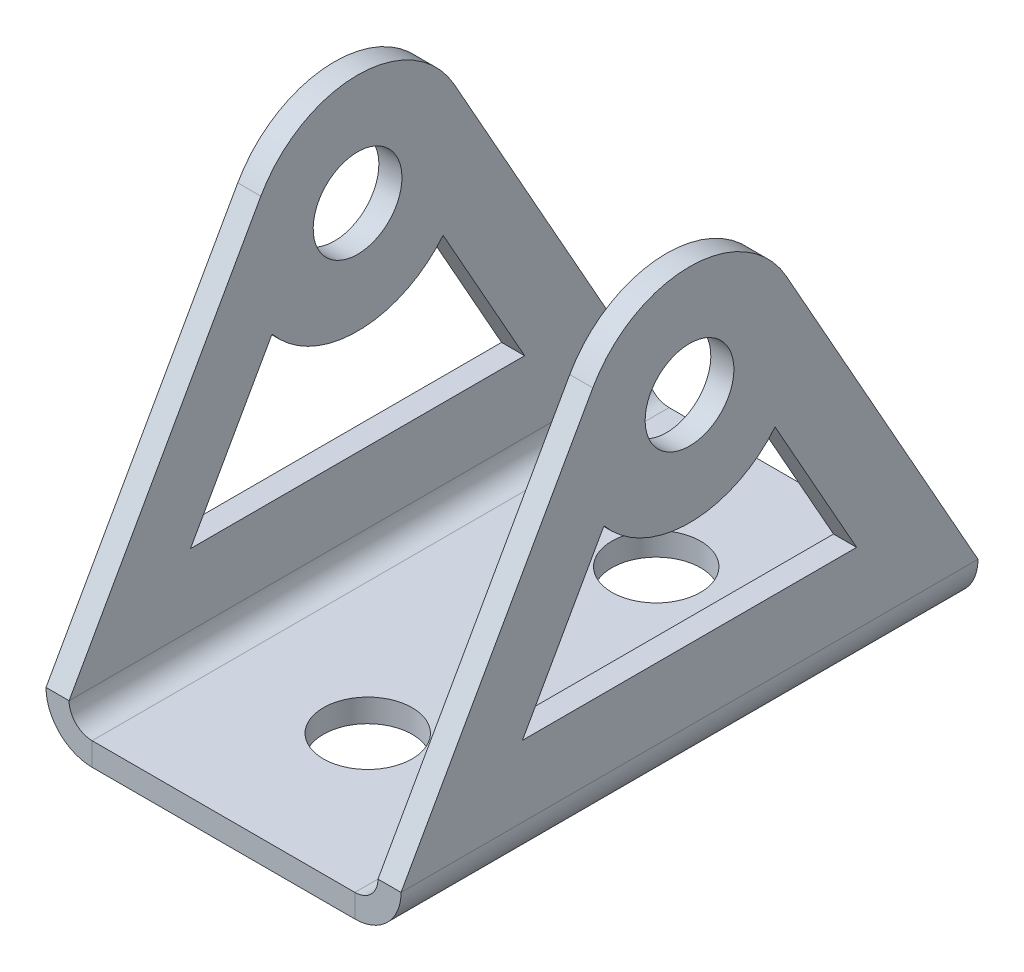
ISO-10303-21;
HEADER;
FILE_DESCRIPTION(('STEP AP214'),'2;1');
FILE_NAME('part.step','',(''),(''),'','','');
FILE_SCHEMA(('AUTOMOTIVE_DESIGN { 1 0 10303 214 1 1 1 1 }'));
ENDSEC;
DATA;
#1=APPLICATION_CONTEXT('core data for automotive mechanical design processes');
#2=APPLICATION_PROTOCOL_DEFINITION('international standard','automotive_design',2000,#1);
#3=PRODUCT_CONTEXT('',#1,'mechanical');
#4=PRODUCT('Part','Part','',(#3));
#5=PRODUCT_RELATED_PRODUCT_CATEGORY('part','',(#4));
#6=PRODUCT_DEFINITION_FORMATION('','',#4);
#7=PRODUCT_DEFINITION_CONTEXT('part definition',#1,'design');
#8=PRODUCT_DEFINITION('design','',#6,#7);
#9=PRODUCT_DEFINITION_SHAPE('','',#8);
#10=(LENGTH_UNIT() NAMED_UNIT(*) SI_UNIT(.MILLI.,.METRE.));
#11=(NAMED_UNIT(*) PLANE_ANGLE_UNIT() SI_UNIT($,.RADIAN.));
#12=(NAMED_UNIT(*) SI_UNIT($,.STERADIAN.) SOLID_ANGLE_UNIT());
#13=UNCERTAINTY_MEASURE_WITH_UNIT(LENGTH_MEASURE(1.E-05),#10,'distance_accuracy_value','');
#14=(GEOMETRIC_REPRESENTATION_CONTEXT(3) GLOBAL_UNCERTAINTY_ASSIGNED_CONTEXT((#13)) GLOBAL_UNIT_ASSIGNED_CONTEXT((#10,
#11,#12)) REPRESENTATION_CONTEXT('',''));
#15=CARTESIAN_POINT('',(0.,0.,0.));
#16=DIRECTION('',(0.,0.,1.));
#17=DIRECTION('',(1.,0.,0.));
#18=AXIS2_PLACEMENT_3D('',#15,#16,#17);
#19=CARTESIAN_POINT('',(0.,-2.6,0.));
#20=DIRECTION('',(0.,-1.,0.));
#21=DIRECTION('',(0.,0.,-1.));
#22=AXIS2_PLACEMENT_3D('',#19,#20,#21);
#23=PLANE('',#22);
#24=CARTESIAN_POINT('',(0.,-2.6,16.25));
#25=DIRECTION('',(0.,1.,0.));
#26=DIRECTION('',(0.,0.,1.));
#27=AXIS2_PLACEMENT_3D('',#24,#25,#26);
#28=CIRCLE('',#27,5.);
#29=CARTESIAN_POINT('',(0.,-2.6,21.25));
#30=VERTEX_POINT('',#29);
#31=EDGE_CURVE('E269',#30,#30,#28,.T.);
#32=ORIENTED_EDGE('',*,*,#31,.T.);
#33=EDGE_LOOP('',(#32));
#34=FACE_BOUND('',#33,.T.);
#35=CARTESIAN_POINT('',(0.,-2.6,-16.25));
#36=DIRECTION('',(0.,1.,0.));
#37=DIRECTION('',(0.,0.,1.));
#38=AXIS2_PLACEMENT_3D('',#35,#36,#37);
#39=CIRCLE('',#38,5.);
#40=CARTESIAN_POINT('',(0.,-2.6,-11.25));
#41=VERTEX_POINT('',#40);
#42=EDGE_CURVE('E277',#41,#41,#39,.T.);
#43=ORIENTED_EDGE('',*,*,#42,.T.);
#44=EDGE_LOOP('',(#43));
#45=FACE_BOUND('',#44,.T.);
#46=DIRECTION('',(1.,0.,0.));
#47=VECTOR('',#46,1.);
#48=CARTESIAN_POINT('',(-20.,-2.6,32.5));
#49=LINE('',#48,#47);
#50=CARTESIAN_POINT('',(-14.8,-2.6,32.5));
#51=VERTEX_POINT('',#50);
#52=CARTESIAN_POINT('',(14.8,-2.6,32.5));
#53=VERTEX_POINT('',#52);
#54=EDGE_CURVE('E13',#51,#53,#49,.T.);
#55=ORIENTED_EDGE('',*,*,#54,.F.);
#56=DIRECTION('',(0.,0.,1.));
#57=VECTOR('',#56,1.);
#58=CARTESIAN_POINT('',(-14.8,-2.6,32.5));
#59=LINE('',#58,#57);
#60=CARTESIAN_POINT('',(-14.8,-2.6,-32.5));
#61=VERTEX_POINT('',#60);
#62=EDGE_CURVE('E444',#51,#61,#59,.F.);
#63=ORIENTED_EDGE('',*,*,#62,.T.);
#64=DIRECTION('',(-1.,0.,0.));
#65=VECTOR('',#64,1.);
#66=CARTESIAN_POINT('',(-20.,-2.6,-32.5));
#67=LINE('',#66,#65);
#68=CARTESIAN_POINT('',(14.8,-2.6,-32.5));
#69=VERTEX_POINT('',#68);
#70=EDGE_CURVE('E134',#69,#61,#67,.T.);
#71=ORIENTED_EDGE('',*,*,#70,.F.);
#72=DIRECTION('',(0.,0.,-1.));
#73=VECTOR('',#72,1.);
#74=CARTESIAN_POINT('',(14.8,-2.6,-32.5));
#75=LINE('',#74,#73);
#76=EDGE_CURVE('E148',#69,#53,#75,.F.);
#77=ORIENTED_EDGE('',*,*,#76,.T.);
#78=EDGE_LOOP('',(#55,#63,#71,#77));
#79=FACE_BOUND('',#78,.T.);
#80=ADVANCED_FACE('F123',(#34,#45,#79),#23,.T.);
#81=CARTESIAN_POINT('',(0.,0.,0.));
#82=DIRECTION('',(0.,-1.,0.));
#83=DIRECTION('',(0.,0.,-1.));
#84=AXIS2_PLACEMENT_3D('',#81,#82,#83);
#85=PLANE('',#84);
#86=CARTESIAN_POINT('',(0.,0.,16.25));
#87=DIRECTION('',(0.,1.,0.));
#88=DIRECTION('',(0.,0.,1.));
#89=AXIS2_PLACEMENT_3D('',#86,#87,#88);
#90=CIRCLE('',#89,5.);
#91=CARTESIAN_POINT('',(0.,0.,21.25));
#92=VERTEX_POINT('',#91);
#93=EDGE_CURVE('E268',#92,#92,#90,.T.);
#94=ORIENTED_EDGE('',*,*,#93,.F.);
#95=EDGE_LOOP('',(#94));
#96=FACE_BOUND('',#95,.T.);
#97=CARTESIAN_POINT('',(0.,0.,-16.25));
#98=DIRECTION('',(0.,1.,0.));
#99=DIRECTION('',(0.,0.,1.));
#100=AXIS2_PLACEMENT_3D('',#97,#98,#99);
#101=CIRCLE('',#100,5.);
#102=CARTESIAN_POINT('',(0.,0.,-11.25));
#103=VERTEX_POINT('',#102);
#104=EDGE_CURVE('E272',#103,#103,#101,.T.);
#105=ORIENTED_EDGE('',*,*,#104,.F.);
#106=EDGE_LOOP('',(#105));
#107=FACE_BOUND('',#106,.T.);
#108=DIRECTION('',(0.,0.,1.));
#109=VECTOR('',#108,1.);
#110=CARTESIAN_POINT('',(-14.8,0.,32.5));
#111=LINE('',#110,#109);
#112=CARTESIAN_POINT('',(-14.8,0.,32.5));
#113=VERTEX_POINT('',#112);
#114=CARTESIAN_POINT('',(-14.8,0.,-32.5));
#115=VERTEX_POINT('',#114);
#116=EDGE_CURVE('E295',#113,#115,#111,.F.);
#117=ORIENTED_EDGE('',*,*,#116,.F.);
#118=DIRECTION('',(1.,0.,0.));
#119=VECTOR('',#118,1.);
#120=CARTESIAN_POINT('',(-20.,0.,32.5));
#121=LINE('',#120,#119);
#122=CARTESIAN_POINT('',(14.8,0.,32.5));
#123=VERTEX_POINT('',#122);
#124=EDGE_CURVE('E130',#113,#123,#121,.T.);
#125=ORIENTED_EDGE('',*,*,#124,.T.);
#126=DIRECTION('',(0.,0.,-1.));
#127=VECTOR('',#126,1.);
#128=CARTESIAN_POINT('',(14.8,0.,-32.5));
#129=LINE('',#128,#127);
#130=CARTESIAN_POINT('',(14.8,0.,-32.5));
#131=VERTEX_POINT('',#130);
#132=EDGE_CURVE('E191',#131,#123,#129,.F.);
#133=ORIENTED_EDGE('',*,*,#132,.F.);
#134=DIRECTION('',(-1.,0.,0.));
#135=VECTOR('',#134,1.);
#136=CARTESIAN_POINT('',(-20.,0.,-32.5));
#137=LINE('',#136,#135);
#138=EDGE_CURVE('E276',#131,#115,#137,.T.);
#139=ORIENTED_EDGE('',*,*,#138,.T.);
#140=EDGE_LOOP('',(#117,#125,#133,#139));
#141=FACE_BOUND('',#140,.T.);
#142=ADVANCED_FACE('F289',(#96,#107,#141),#85,.F.);
#143=CARTESIAN_POINT('',(-20.,-2.6,32.5));
#144=DIRECTION('',(0.,0.,1.));
#145=DIRECTION('',(1.,0.,0.));
#146=AXIS2_PLACEMENT_3D('',#143,#144,#145);
#147=PLANE('',#146);
#148=ORIENTED_EDGE('',*,*,#124,.F.);
#149=DIRECTION('',(0.,-1.,0.));
#150=VECTOR('',#149,1.);
#151=CARTESIAN_POINT('',(-14.8,0.,32.5));
#152=LINE('',#151,#150);
#153=EDGE_CURVE('E449',#113,#51,#152,.T.);
#154=ORIENTED_EDGE('',*,*,#153,.T.);
#155=ORIENTED_EDGE('',*,*,#54,.T.);
#156=DIRECTION('',(0.,-1.,0.));
#157=VECTOR('',#156,1.);
#158=CARTESIAN_POINT('',(14.8,0.,32.5));
#159=LINE('',#158,#157);
#160=EDGE_CURVE('E264',#123,#53,#159,.T.);
#161=ORIENTED_EDGE('',*,*,#160,.F.);
#162=EDGE_LOOP('',(#148,#154,#155,#161));
#163=FACE_BOUND('',#162,.T.);
#164=ADVANCED_FACE('F299',(#163),#147,.T.);
#165=CARTESIAN_POINT('',(-20.,-2.6,-32.5));
#166=DIRECTION('',(0.,0.,-1.));
#167=DIRECTION('',(-1.,0.,0.));
#168=AXIS2_PLACEMENT_3D('',#165,#166,#167);
#169=PLANE('',#168);
#170=DIRECTION('',(0.,-1.,0.));
#171=VECTOR('',#170,1.);
#172=CARTESIAN_POINT('',(-14.8,0.,-32.5));
#173=LINE('',#172,#171);
#174=EDGE_CURVE('E176',#115,#61,#173,.T.);
#175=ORIENTED_EDGE('',*,*,#174,.F.);
#176=ORIENTED_EDGE('',*,*,#138,.F.);
#177=DIRECTION('',(0.,-1.,0.));
#178=VECTOR('',#177,1.);
#179=CARTESIAN_POINT('',(14.8,0.,-32.5));
#180=LINE('',#179,#178);
#181=EDGE_CURVE('E188',#131,#69,#180,.T.);
#182=ORIENTED_EDGE('',*,*,#181,.T.);
#183=ORIENTED_EDGE('',*,*,#70,.T.);
#184=EDGE_LOOP('',(#175,#176,#182,#183));
#185=FACE_BOUND('',#184,.T.);
#186=ADVANCED_FACE('F121',(#185),#169,.T.);
#187=CARTESIAN_POINT('',(0.,-2.6,-16.25));
#188=DIRECTION('',(0.,1.,0.));
#189=DIRECTION('',(0.,0.,1.));
#190=AXIS2_PLACEMENT_3D('',#187,#188,#189);
#191=CYLINDRICAL_SURFACE('',#190,5.);
#192=ORIENTED_EDGE('',*,*,#42,.F.);
#193=EDGE_LOOP('',(#192));
#194=FACE_BOUND('',#193,.T.);
#195=ORIENTED_EDGE('',*,*,#104,.T.);
#196=EDGE_LOOP('',(#195));
#197=FACE_BOUND('',#196,.T.);
#198=ADVANCED_FACE('F302',(#194,#197),#191,.F.);
#199=CARTESIAN_POINT('',(0.,-2.6,16.25));
#200=DIRECTION('',(0.,1.,0.));
#201=DIRECTION('',(0.,0.,1.));
#202=AXIS2_PLACEMENT_3D('',#199,#200,#201);
#203=CYLINDRICAL_SURFACE('',#202,5.);
#204=ORIENTED_EDGE('',*,*,#31,.F.);
#205=EDGE_LOOP('',(#204));
#206=FACE_BOUND('',#205,.T.);
#207=ORIENTED_EDGE('',*,*,#93,.T.);
#208=EDGE_LOOP('',(#207));
#209=FACE_BOUND('',#208,.T.);
#210=ADVANCED_FACE('F320',(#206,#209),#203,.F.);
#211=CARTESIAN_POINT('',(14.8,2.6,32.5));
#212=DIRECTION('',(0.,0.,1.));
#213=DIRECTION('',(1.,0.,0.));
#214=AXIS2_PLACEMENT_3D('',#211,#212,#213);
#215=PLANE('',#214);
#216=DIRECTION('',(1.,0.,0.));
#217=VECTOR('',#216,1.);
#218=CARTESIAN_POINT('',(17.4,2.59999999999999,32.5));
#219=LINE('',#218,#217);
#220=CARTESIAN_POINT('',(20.,2.59999999999998,32.5));
#221=VERTEX_POINT('',#220);
#222=CARTESIAN_POINT('',(17.4,2.59999999999999,32.5));
#223=VERTEX_POINT('',#222);
#224=EDGE_CURVE('E297',#221,#223,#219,.F.);
#225=ORIENTED_EDGE('',*,*,#224,.T.);
#226=CARTESIAN_POINT('',(14.8,2.6,32.5));
#227=DIRECTION('',(0.,0.,-1.));
#228=DIRECTION('',(-1.,0.,0.));
#229=AXIS2_PLACEMENT_3D('',#226,#227,#228);
#230=CIRCLE('',#229,2.6);
#231=EDGE_CURVE('E172',#123,#223,#230,.F.);
#232=ORIENTED_EDGE('',*,*,#231,.F.);
#233=ORIENTED_EDGE('',*,*,#160,.T.);
#234=CARTESIAN_POINT('',(14.8,2.6,32.5));
#235=DIRECTION('',(0.,0.,-1.));
#236=DIRECTION('',(-1.,0.,0.));
#237=AXIS2_PLACEMENT_3D('',#234,#235,#236);
#238=CIRCLE('',#237,5.2);
#239=EDGE_CURVE('E256',#53,#221,#238,.F.);
#240=ORIENTED_EDGE('',*,*,#239,.T.);
#241=EDGE_LOOP('',(#225,#232,#233,#240));
#242=FACE_BOUND('',#241,.T.);
#243=ADVANCED_FACE('F294',(#242),#215,.T.);
#244=CARTESIAN_POINT('',(14.8,2.6,-32.5));
#245=DIRECTION('',(0.,0.,1.));
#246=DIRECTION('',(1.,0.,0.));
#247=AXIS2_PLACEMENT_3D('',#244,#245,#246);
#248=PLANE('',#247);
#249=CARTESIAN_POINT('',(14.8,2.6,-32.5));
#250=DIRECTION('',(0.,0.,-1.));
#251=DIRECTION('',(-1.,0.,0.));
#252=AXIS2_PLACEMENT_3D('',#249,#250,#251);
#253=CIRCLE('',#252,2.6);
#254=CARTESIAN_POINT('',(17.4,2.59999999999999,-32.5));
#255=VERTEX_POINT('',#254);
#256=EDGE_CURVE('E173',#255,#131,#253,.T.);
#257=ORIENTED_EDGE('',*,*,#256,.F.);
#258=DIRECTION('',(1.,0.,0.));
#259=VECTOR('',#258,1.);
#260=CARTESIAN_POINT('',(20.,2.59999999999999,-32.5));
#261=LINE('',#260,#259);
#262=CARTESIAN_POINT('',(20.,2.59999999999999,-32.5));
#263=VERTEX_POINT('',#262);
#264=EDGE_CURVE('E189',#263,#255,#261,.F.);
#265=ORIENTED_EDGE('',*,*,#264,.F.);
#266=CARTESIAN_POINT('',(14.8,2.6,-32.5));
#267=DIRECTION('',(0.,0.,-1.));
#268=DIRECTION('',(-1.,0.,0.));
#269=AXIS2_PLACEMENT_3D('',#266,#267,#268);
#270=CIRCLE('',#269,5.2);
#271=EDGE_CURVE('E259',#263,#69,#270,.T.);
#272=ORIENTED_EDGE('',*,*,#271,.T.);
#273=ORIENTED_EDGE('',*,*,#181,.F.);
#274=EDGE_LOOP('',(#257,#265,#272,#273));
#275=FACE_BOUND('',#274,.T.);
#276=ADVANCED_FACE('F183',(#275),#248,.F.);
#277=CARTESIAN_POINT('',(14.8,2.6,-32.5));
#278=DIRECTION('',(0.,0.,-1.));
#279=DIRECTION('',(1.,0.,0.));
#280=AXIS2_PLACEMENT_3D('',#277,#278,#279);
#281=CYLINDRICAL_SURFACE('',#280,5.2);
#282=ORIENTED_EDGE('',*,*,#76,.F.);
#283=ORIENTED_EDGE('',*,*,#271,.F.);
#284=DIRECTION('',(0.,0.,-1.));
#285=VECTOR('',#284,1.);
#286=CARTESIAN_POINT('',(20.,2.59999999999998,0.));
#287=LINE('',#286,#285);
#288=EDGE_CURVE('E179',#221,#263,#287,.T.);
#289=ORIENTED_EDGE('',*,*,#288,.F.);
#290=ORIENTED_EDGE('',*,*,#239,.F.);
#291=EDGE_LOOP('',(#282,#283,#289,#290));
#292=FACE_BOUND('',#291,.T.);
#293=ADVANCED_FACE('F322',(#292),#281,.T.);
#294=CARTESIAN_POINT('',(14.8,2.6,-32.5));
#295=DIRECTION('',(0.,0.,-1.));
#296=DIRECTION('',(1.,0.,0.));
#297=AXIS2_PLACEMENT_3D('',#294,#295,#296);
#298=CYLINDRICAL_SURFACE('',#297,2.6);
#299=ORIENTED_EDGE('',*,*,#132,.T.);
#300=ORIENTED_EDGE('',*,*,#231,.T.);
#301=DIRECTION('',(0.,0.,1.));
#302=VECTOR('',#301,1.);
#303=CARTESIAN_POINT('',(17.4,2.59999999999999,32.5));
#304=LINE('',#303,#302);
#305=EDGE_CURVE('E170',#223,#255,#304,.F.);
#306=ORIENTED_EDGE('',*,*,#305,.T.);
#307=ORIENTED_EDGE('',*,*,#256,.T.);
#308=EDGE_LOOP('',(#299,#300,#306,#307));
#309=FACE_BOUND('',#308,.T.);
#310=ADVANCED_FACE('F168',(#309),#298,.F.);
#311=CARTESIAN_POINT('',(20.0000000000001,34.9,0.));
#312=DIRECTION('',(1.,0.,0.));
#313=DIRECTION('',(0.,1.,0.));
#314=AXIS2_PLACEMENT_3D('',#311,#312,#313);
#315=PLANE('',#314);
#316=DIRECTION('',(0.,-0.871678199606987,0.49007868381508));
#317=VECTOR('',#316,1.);
#318=CARTESIAN_POINT('',(20.,10.6,18.8245065944115));
#319=LINE('',#318,#317);
#320=CARTESIAN_POINT('',(20.0000000000001,26.9399267777804,9.6378023582611));
#321=VERTEX_POINT('',#320);
#322=CARTESIAN_POINT('',(20.,10.6,18.8245065944115));
#323=VERTEX_POINT('',#322);
#324=EDGE_CURVE('E235',#321,#323,#319,.T.);
#325=ORIENTED_EDGE('',*,*,#324,.F.);
#326=CARTESIAN_POINT('',(20.0000000000001,34.9,0.));
#327=DIRECTION('',(1.,0.,0.));
#328=DIRECTION('',(0.,1.,0.));
#329=AXIS2_PLACEMENT_3D('',#326,#327,#328);
#330=CIRCLE('',#329,12.5);
#331=CARTESIAN_POINT('',(20.0000000000001,26.9399267777804,-9.6378023582611));
#332=VERTEX_POINT('',#331);
#333=EDGE_CURVE('E231',#332,#321,#330,.F.);
#334=ORIENTED_EDGE('',*,*,#333,.F.);
#335=DIRECTION('',(0.,0.871678199606987,0.49007868381508));
#336=VECTOR('',#335,1.);
#337=CARTESIAN_POINT('',(20.,10.6,-18.8245065944115));
#338=LINE('',#337,#336);
#339=CARTESIAN_POINT('',(20.,10.6,-18.8245065944115));
#340=VERTEX_POINT('',#339);
#341=EDGE_CURVE('E228',#340,#332,#338,.T.);
#342=ORIENTED_EDGE('',*,*,#341,.F.);
#343=DIRECTION('',(0.,0.,-1.));
#344=VECTOR('',#343,1.);
#345=CARTESIAN_POINT('',(20.,10.6,-18.8245065944115));
#346=LINE('',#345,#344);
#347=EDGE_CURVE('E227',#323,#340,#346,.T.);
#348=ORIENTED_EDGE('',*,*,#347,.F.);
#349=EDGE_LOOP('',(#325,#334,#342,#348));
#350=FACE_BOUND('',#349,.T.);
#351=CARTESIAN_POINT('',(20.0000000000001,34.9,0.));
#352=DIRECTION('',(1.,0.,0.));
#353=DIRECTION('',(0.,1.,0.));
#354=AXIS2_PLACEMENT_3D('',#351,#352,#353);
#355=CIRCLE('',#354,5.);
#356=CARTESIAN_POINT('',(20.0000000000001,39.9,0.));
#357=VERTEX_POINT('',#356);
#358=EDGE_CURVE('E249',#357,#357,#355,.T.);
#359=ORIENTED_EDGE('',*,*,#358,.F.);
#360=EDGE_LOOP('',(#359));
#361=FACE_BOUND('',#360,.T.);
#362=DIRECTION('',(0.,0.871678199606987,-0.49007868381508));
#363=VECTOR('',#362,1.);
#364=CARTESIAN_POINT('',(20.0000000000001,41.0259835476885,10.8959774950873));
#365=LINE('',#364,#363);
#366=CARTESIAN_POINT('',(20.0000000000001,41.0259835476885,10.8959774950873));
#367=VERTEX_POINT('',#366);
#368=EDGE_CURVE('E468',#367,#221,#365,.F.);
#369=ORIENTED_EDGE('',*,*,#368,.T.);
#370=ORIENTED_EDGE('',*,*,#288,.T.);
#371=DIRECTION('',(0.,-0.871678199606987,-0.49007868381508));
#372=VECTOR('',#371,1.);
#373=CARTESIAN_POINT('',(20.0000000000001,41.0259835476885,-10.8959774950873));
#374=LINE('',#373,#372);
#375=CARTESIAN_POINT('',(20.0000000000001,41.0259835476885,-10.8959774950873));
#376=VERTEX_POINT('',#375);
#377=EDGE_CURVE('E205',#263,#376,#374,.F.);
#378=ORIENTED_EDGE('',*,*,#377,.T.);
#379=CARTESIAN_POINT('',(20.0000000000001,34.9,0.));
#380=DIRECTION('',(1.,0.,0.));
#381=DIRECTION('',(0.,1.,0.));
#382=AXIS2_PLACEMENT_3D('',#379,#380,#381);
#383=CIRCLE('',#382,12.5);
#384=EDGE_CURVE('E472',#376,#367,#383,.T.);
#385=ORIENTED_EDGE('',*,*,#384,.T.);
#386=EDGE_LOOP('',(#369,#370,#378,#385));
#387=FACE_BOUND('',#386,.T.);
#388=ADVANCED_FACE('F328',(#350,#361,#387),#315,.T.);
#389=CARTESIAN_POINT('',(17.4000000000001,34.9,0.));
#390=DIRECTION('',(1.,0.,0.));
#391=DIRECTION('',(0.,1.,0.));
#392=AXIS2_PLACEMENT_3D('',#389,#390,#391);
#393=PLANE('',#392);
#394=CARTESIAN_POINT('',(17.4000000000001,34.9,0.));
#395=DIRECTION('',(1.,0.,0.));
#396=DIRECTION('',(0.,1.,0.));
#397=AXIS2_PLACEMENT_3D('',#394,#395,#396);
#398=CIRCLE('',#397,5.);
#399=CARTESIAN_POINT('',(17.4000000000001,39.9,0.));
#400=VERTEX_POINT('',#399);
#401=EDGE_CURVE('E251',#400,#400,#398,.T.);
#402=ORIENTED_EDGE('',*,*,#401,.T.);
#403=EDGE_LOOP('',(#402));
#404=FACE_BOUND('',#403,.T.);
#405=CARTESIAN_POINT('',(17.4000000000001,34.9,0.));
#406=DIRECTION('',(1.,0.,0.));
#407=DIRECTION('',(0.,1.,0.));
#408=AXIS2_PLACEMENT_3D('',#405,#406,#407);
#409=CIRCLE('',#408,12.5);
#410=CARTESIAN_POINT('',(17.4000000000001,26.9399267777805,-9.6378023582611));
#411=VERTEX_POINT('',#410);
#412=CARTESIAN_POINT('',(17.4000000000001,26.9399267777805,9.6378023582611));
#413=VERTEX_POINT('',#412);
#414=EDGE_CURVE('E250',#411,#413,#409,.F.);
#415=ORIENTED_EDGE('',*,*,#414,.T.);
#416=DIRECTION('',(0.,0.871678199606987,-0.49007868381508));
#417=VECTOR('',#416,1.);
#418=CARTESIAN_POINT('',(17.4000000000001,37.1053540771679,3.92255189823144));
#419=LINE('',#418,#417);
#420=CARTESIAN_POINT('',(17.4,10.6,18.8245065944115));
#421=VERTEX_POINT('',#420);
#422=EDGE_CURVE('E241',#413,#421,#419,.F.);
#423=ORIENTED_EDGE('',*,*,#422,.T.);
#424=DIRECTION('',(0.,0.,1.));
#425=VECTOR('',#424,1.);
#426=CARTESIAN_POINT('',(17.4,10.6,0.));
#427=LINE('',#426,#425);
#428=CARTESIAN_POINT('',(17.4,10.6,-18.8245065944115));
#429=VERTEX_POINT('',#428);
#430=EDGE_CURVE('E242',#421,#429,#427,.F.);
#431=ORIENTED_EDGE('',*,*,#430,.T.);
#432=DIRECTION('',(0.,-0.871678199606987,-0.49007868381508));
#433=VECTOR('',#432,1.);
#434=CARTESIAN_POINT('',(17.4000000000001,37.1053540771679,-3.92255189823144));
#435=LINE('',#434,#433);
#436=EDGE_CURVE('E236',#429,#411,#435,.F.);
#437=ORIENTED_EDGE('',*,*,#436,.T.);
#438=EDGE_LOOP('',(#415,#423,#431,#437));
#439=FACE_BOUND('',#438,.T.);
#440=ORIENTED_EDGE('',*,*,#305,.F.);
#441=DIRECTION('',(0.,-0.871678199606987,0.49007868381508));
#442=VECTOR('',#441,1.);
#443=CARTESIAN_POINT('',(17.4,2.6,32.5));
#444=LINE('',#443,#442);
#445=CARTESIAN_POINT('',(17.4000000000001,41.0259835476885,10.8959774950873));
#446=VERTEX_POINT('',#445);
#447=EDGE_CURVE('E211',#446,#223,#444,.T.);
#448=ORIENTED_EDGE('',*,*,#447,.F.);
#449=CARTESIAN_POINT('',(17.4000000000001,34.9,0.));
#450=DIRECTION('',(1.,0.,0.));
#451=DIRECTION('',(0.,1.,0.));
#452=AXIS2_PLACEMENT_3D('',#449,#450,#451);
#453=CIRCLE('',#452,12.5);
#454=CARTESIAN_POINT('',(17.4000000000001,41.0259835476885,-10.8959774950873));
#455=VERTEX_POINT('',#454);
#456=EDGE_CURVE('E208',#455,#446,#453,.T.);
#457=ORIENTED_EDGE('',*,*,#456,.F.);
#458=DIRECTION('',(0.,0.871678199606987,0.49007868381508));
#459=VECTOR('',#458,1.);
#460=CARTESIAN_POINT('',(17.4,2.6,-32.5));
#461=LINE('',#460,#459);
#462=EDGE_CURVE('E200',#255,#455,#461,.T.);
#463=ORIENTED_EDGE('',*,*,#462,.F.);
#464=EDGE_LOOP('',(#440,#448,#457,#463));
#465=FACE_BOUND('',#464,.T.);
#466=ADVANCED_FACE('F206',(#404,#439,#465),#393,.F.);
#467=CARTESIAN_POINT('',(20.,2.59999999999999,-32.5));
#468=DIRECTION('',(0.,-0.49007868381508,0.871678199606987));
#469=DIRECTION('',(0.,-0.871678199606987,-0.49007868381508));
#470=AXIS2_PLACEMENT_3D('',#467,#468,#469);
#471=PLANE('',#470);
#472=ORIENTED_EDGE('',*,*,#462,.T.);
#473=DIRECTION('',(-1.,0.,0.));
#474=VECTOR('',#473,1.);
#475=CARTESIAN_POINT('',(20.0000000000001,41.0259835476885,-10.8959774950873));
#476=LINE('',#475,#474);
#477=EDGE_CURVE('E201',#376,#455,#476,.T.);
#478=ORIENTED_EDGE('',*,*,#477,.F.);
#479=ORIENTED_EDGE('',*,*,#377,.F.);
#480=ORIENTED_EDGE('',*,*,#264,.T.);
#481=EDGE_LOOP('',(#472,#478,#479,#480));
#482=FACE_BOUND('',#481,.T.);
#483=ADVANCED_FACE('F198',(#482),#471,.F.);
#484=CARTESIAN_POINT('',(20.0000000000001,34.9,0.));
#485=DIRECTION('',(-1.,0.,0.));
#486=DIRECTION('',(0.,-1.,0.));
#487=AXIS2_PLACEMENT_3D('',#484,#485,#486);
#488=CYLINDRICAL_SURFACE('',#487,12.5);
#489=ORIENTED_EDGE('',*,*,#456,.T.);
#490=DIRECTION('',(-1.,0.,0.));
#491=VECTOR('',#490,1.);
#492=CARTESIAN_POINT('',(20.0000000000001,41.0259835476885,10.8959774950873));
#493=LINE('',#492,#491);
#494=EDGE_CURVE('E461',#367,#446,#493,.T.);
#495=ORIENTED_EDGE('',*,*,#494,.F.);
#496=ORIENTED_EDGE('',*,*,#384,.F.);
#497=ORIENTED_EDGE('',*,*,#477,.T.);
#498=EDGE_LOOP('',(#489,#495,#496,#497));
#499=FACE_BOUND('',#498,.T.);
#500=ADVANCED_FACE('F331',(#499),#488,.T.);
#501=CARTESIAN_POINT('',(20.,2.59999999999999,32.5));
#502=DIRECTION('',(0.,-0.49007868381508,-0.871678199606987));
#503=DIRECTION('',(0.,0.871678199606987,-0.49007868381508));
#504=AXIS2_PLACEMENT_3D('',#501,#502,#503);
#505=PLANE('',#504);
#506=ORIENTED_EDGE('',*,*,#447,.T.);
#507=ORIENTED_EDGE('',*,*,#224,.F.);
#508=ORIENTED_EDGE('',*,*,#368,.F.);
#509=ORIENTED_EDGE('',*,*,#494,.T.);
#510=EDGE_LOOP('',(#506,#507,#508,#509));
#511=FACE_BOUND('',#510,.T.);
#512=ADVANCED_FACE('F340',(#511),#505,.F.);
#513=CARTESIAN_POINT('',(20.0000000000001,34.9,0.));
#514=DIRECTION('',(-1.,0.,0.));
#515=DIRECTION('',(0.,-1.,0.));
#516=AXIS2_PLACEMENT_3D('',#513,#514,#515);
#517=CYLINDRICAL_SURFACE('',#516,12.5);
#518=ORIENTED_EDGE('',*,*,#414,.F.);
#519=DIRECTION('',(-1.,0.,0.));
#520=VECTOR('',#519,1.);
#521=CARTESIAN_POINT('',(20.0000000000001,26.9399267777804,-9.6378023582611));
#522=LINE('',#521,#520);
#523=EDGE_CURVE('E224',#332,#411,#522,.T.);
#524=ORIENTED_EDGE('',*,*,#523,.F.);
#525=ORIENTED_EDGE('',*,*,#333,.T.);
#526=DIRECTION('',(-1.,0.,0.));
#527=VECTOR('',#526,1.);
#528=CARTESIAN_POINT('',(20.0000000000001,26.9399267777804,9.6378023582611));
#529=LINE('',#528,#527);
#530=EDGE_CURVE('E207',#321,#413,#529,.T.);
#531=ORIENTED_EDGE('',*,*,#530,.T.);
#532=EDGE_LOOP('',(#518,#524,#525,#531));
#533=FACE_BOUND('',#532,.T.);
#534=ADVANCED_FACE('F342',(#533),#517,.T.);
#535=CARTESIAN_POINT('',(20.,10.6,18.8245065944115));
#536=DIRECTION('',(0.,-0.49007868381508,-0.871678199606987));
#537=DIRECTION('',(0.,0.871678199606987,-0.49007868381508));
#538=AXIS2_PLACEMENT_3D('',#535,#536,#537);
#539=PLANE('',#538);
#540=ORIENTED_EDGE('',*,*,#422,.F.);
#541=ORIENTED_EDGE('',*,*,#530,.F.);
#542=ORIENTED_EDGE('',*,*,#324,.T.);
#543=DIRECTION('',(1.,0.,0.));
#544=VECTOR('',#543,1.);
#545=CARTESIAN_POINT('',(20.,10.6,18.8245065944115));
#546=LINE('',#545,#544);
#547=EDGE_CURVE('E212',#323,#421,#546,.F.);
#548=ORIENTED_EDGE('',*,*,#547,.T.);
#549=EDGE_LOOP('',(#540,#541,#542,#548));
#550=FACE_BOUND('',#549,.T.);
#551=ADVANCED_FACE('F352',(#550),#539,.T.);
#552=CARTESIAN_POINT('',(20.,10.6,-18.8245065944115));
#553=DIRECTION('',(0.,1.,0.));
#554=DIRECTION('',(-1.,0.,0.));
#555=AXIS2_PLACEMENT_3D('',#552,#553,#554);
#556=PLANE('',#555);
#557=ORIENTED_EDGE('',*,*,#430,.F.);
#558=ORIENTED_EDGE('',*,*,#547,.F.);
#559=ORIENTED_EDGE('',*,*,#347,.T.);
#560=DIRECTION('',(1.,0.,0.));
#561=VECTOR('',#560,1.);
#562=CARTESIAN_POINT('',(20.,10.6,-18.8245065944115));
#563=LINE('',#562,#561);
#564=EDGE_CURVE('E219',#340,#429,#563,.F.);
#565=ORIENTED_EDGE('',*,*,#564,.T.);
#566=EDGE_LOOP('',(#557,#558,#559,#565));
#567=FACE_BOUND('',#566,.T.);
#568=ADVANCED_FACE('F353',(#567),#556,.T.);
#569=CARTESIAN_POINT('',(20.,10.6,-18.8245065944115));
#570=DIRECTION('',(0.,-0.49007868381508,0.871678199606987));
#571=DIRECTION('',(0.,-0.871678199606987,-0.49007868381508));
#572=AXIS2_PLACEMENT_3D('',#569,#570,#571);
#573=PLANE('',#572);
#574=ORIENTED_EDGE('',*,*,#436,.F.);
#575=ORIENTED_EDGE('',*,*,#564,.F.);
#576=ORIENTED_EDGE('',*,*,#341,.T.);
#577=ORIENTED_EDGE('',*,*,#523,.T.);
#578=EDGE_LOOP('',(#574,#575,#576,#577));
#579=FACE_BOUND('',#578,.T.);
#580=ADVANCED_FACE('F358',(#579),#573,.T.);
#581=CARTESIAN_POINT('',(20.0000000000001,34.9,0.));
#582=DIRECTION('',(-1.,0.,0.));
#583=DIRECTION('',(0.,-1.,0.));
#584=AXIS2_PLACEMENT_3D('',#581,#582,#583);
#585=CYLINDRICAL_SURFACE('',#584,5.);
#586=ORIENTED_EDGE('',*,*,#358,.T.);
#587=EDGE_LOOP('',(#586));
#588=FACE_BOUND('',#587,.T.);
#589=ORIENTED_EDGE('',*,*,#401,.F.);
#590=EDGE_LOOP('',(#589));
#591=FACE_BOUND('',#590,.T.);
#592=ADVANCED_FACE('F361',(#588,#591),#585,.F.);
#593=CARTESIAN_POINT('',(-14.8,2.6,-32.5));
#594=DIRECTION('',(0.,0.,-1.));
#595=DIRECTION('',(-1.,0.,0.));
#596=AXIS2_PLACEMENT_3D('',#593,#594,#595);
#597=PLANE('',#596);
#598=DIRECTION('',(1.,0.,0.));
#599=VECTOR('',#598,1.);
#600=CARTESIAN_POINT('',(-17.4,2.59999999999999,-32.5));
#601=LINE('',#600,#599);
#602=CARTESIAN_POINT('',(-20.,2.59999999999998,-32.5));
#603=VERTEX_POINT('',#602);
#604=CARTESIAN_POINT('',(-17.4,2.59999999999999,-32.5));
#605=VERTEX_POINT('',#604);
#606=EDGE_CURVE('E625',#603,#605,#601,.T.);
#607=ORIENTED_EDGE('',*,*,#606,.T.);
#608=CARTESIAN_POINT('',(-14.8,2.6,-32.5));
#609=DIRECTION('',(0.,0.,1.));
#610=DIRECTION('',(1.,0.,0.));
#611=AXIS2_PLACEMENT_3D('',#608,#609,#610);
#612=CIRCLE('',#611,2.6);
#613=EDGE_CURVE('E453',#115,#605,#612,.F.);
#614=ORIENTED_EDGE('',*,*,#613,.F.);
#615=ORIENTED_EDGE('',*,*,#174,.T.);
#616=CARTESIAN_POINT('',(-14.8,2.6,-32.5));
#617=DIRECTION('',(0.,0.,1.));
#618=DIRECTION('',(1.,0.,0.));
#619=AXIS2_PLACEMENT_3D('',#616,#617,#618);
#620=CIRCLE('',#619,5.2);
#621=EDGE_CURVE('E448',#61,#603,#620,.F.);
#622=ORIENTED_EDGE('',*,*,#621,.T.);
#623=EDGE_LOOP('',(#607,#614,#615,#622));
#624=FACE_BOUND('',#623,.T.);
#625=ADVANCED_FACE('F368',(#624),#597,.T.);
#626=CARTESIAN_POINT('',(-14.8,2.6,32.5));
#627=DIRECTION('',(0.,0.,-1.));
#628=DIRECTION('',(-1.,0.,0.));
#629=AXIS2_PLACEMENT_3D('',#626,#627,#628);
#630=PLANE('',#629);
#631=CARTESIAN_POINT('',(-14.8,2.6,32.5));
#632=DIRECTION('',(0.,0.,1.));
#633=DIRECTION('',(1.,0.,0.));
#634=AXIS2_PLACEMENT_3D('',#631,#632,#633);
#635=CIRCLE('',#634,2.6);
#636=CARTESIAN_POINT('',(-17.4,2.59999999999999,32.5));
#637=VERTEX_POINT('',#636);
#638=EDGE_CURVE('E460',#637,#113,#635,.T.);
#639=ORIENTED_EDGE('',*,*,#638,.F.);
#640=DIRECTION('',(1.,0.,0.));
#641=VECTOR('',#640,1.);
#642=CARTESIAN_POINT('',(-20.,2.59999999999999,32.5));
#643=LINE('',#642,#641);
#644=CARTESIAN_POINT('',(-20.,2.59999999999999,32.5));
#645=VERTEX_POINT('',#644);
#646=EDGE_CURVE('E458',#645,#637,#643,.T.);
#647=ORIENTED_EDGE('',*,*,#646,.F.);
#648=CARTESIAN_POINT('',(-14.8,2.6,32.5));
#649=DIRECTION('',(0.,0.,1.));
#650=DIRECTION('',(1.,0.,0.));
#651=AXIS2_PLACEMENT_3D('',#648,#649,#650);
#652=CIRCLE('',#651,5.2);
#653=EDGE_CURVE('E450',#645,#51,#652,.T.);
#654=ORIENTED_EDGE('',*,*,#653,.T.);
#655=ORIENTED_EDGE('',*,*,#153,.F.);
#656=EDGE_LOOP('',(#639,#647,#654,#655));
#657=FACE_BOUND('',#656,.T.);
#658=ADVANCED_FACE('F366',(#657),#630,.F.);
#659=CARTESIAN_POINT('',(-14.8,2.6,32.5));
#660=DIRECTION('',(0.,0.,1.));
#661=DIRECTION('',(-1.,0.,0.));
#662=AXIS2_PLACEMENT_3D('',#659,#660,#661);
#663=CYLINDRICAL_SURFACE('',#662,5.2);
#664=ORIENTED_EDGE('',*,*,#62,.F.);
#665=ORIENTED_EDGE('',*,*,#653,.F.);
#666=DIRECTION('',(0.,0.,1.));
#667=VECTOR('',#666,1.);
#668=CARTESIAN_POINT('',(-20.,2.59999999999998,0.));
#669=LINE('',#668,#667);
#670=EDGE_CURVE('E435',#603,#645,#669,.T.);
#671=ORIENTED_EDGE('',*,*,#670,.F.);
#672=ORIENTED_EDGE('',*,*,#621,.F.);
#673=EDGE_LOOP('',(#664,#665,#671,#672));
#674=FACE_BOUND('',#673,.T.);
#675=ADVANCED_FACE('F371',(#674),#663,.T.);
#676=CARTESIAN_POINT('',(-14.8,2.6,32.5));
#677=DIRECTION('',(0.,0.,1.));
#678=DIRECTION('',(-1.,0.,0.));
#679=AXIS2_PLACEMENT_3D('',#676,#677,#678);
#680=CYLINDRICAL_SURFACE('',#679,2.6);
#681=ORIENTED_EDGE('',*,*,#116,.T.);
#682=ORIENTED_EDGE('',*,*,#613,.T.);
#683=DIRECTION('',(0.,0.,-1.));
#684=VECTOR('',#683,1.);
#685=CARTESIAN_POINT('',(-17.4,2.59999999999999,-32.5));
#686=LINE('',#685,#684);
#687=EDGE_CURVE('E440',#605,#637,#686,.F.);
#688=ORIENTED_EDGE('',*,*,#687,.T.);
#689=ORIENTED_EDGE('',*,*,#638,.T.);
#690=EDGE_LOOP('',(#681,#682,#688,#689));
#691=FACE_BOUND('',#690,.T.);
#692=ADVANCED_FACE('F376',(#691),#680,.F.);
#693=CARTESIAN_POINT('',(-20.0000000000001,34.9,0.));
#694=DIRECTION('',(-1.,0.,0.));
#695=DIRECTION('',(0.,1.,0.));
#696=AXIS2_PLACEMENT_3D('',#693,#694,#695);
#697=PLANE('',#696);
#698=CARTESIAN_POINT('',(-20.0000000000001,34.9,0.));
#699=DIRECTION('',(-1.,0.,0.));
#700=DIRECTION('',(0.,-1.,0.));
#701=AXIS2_PLACEMENT_3D('',#698,#699,#700);
#702=CIRCLE('',#701,5.);
#703=CARTESIAN_POINT('',(-20.0000000000001,29.9,0.));
#704=VERTEX_POINT('',#703);
#705=EDGE_CURVE('E430',#704,#704,#702,.F.);
#706=ORIENTED_EDGE('',*,*,#705,.T.);
#707=EDGE_LOOP('',(#706));
#708=FACE_BOUND('',#707,.T.);
#709=CARTESIAN_POINT('',(-20.0000000000001,34.9,0.));
#710=DIRECTION('',(-1.,0.,0.));
#711=DIRECTION('',(0.,-1.,0.));
#712=AXIS2_PLACEMENT_3D('',#709,#710,#711);
#713=CIRCLE('',#712,12.5);
#714=CARTESIAN_POINT('',(-20.0000000000001,26.9399267777804,-9.6378023582611));
#715=VERTEX_POINT('',#714);
#716=CARTESIAN_POINT('',(-20.0000000000001,26.9399267777804,9.6378023582611));
#717=VERTEX_POINT('',#716);
#718=EDGE_CURVE('E580',#715,#717,#713,.T.);
#719=ORIENTED_EDGE('',*,*,#718,.T.);
#720=DIRECTION('',(0.,0.871678199606987,-0.49007868381508));
#721=VECTOR('',#720,1.);
#722=CARTESIAN_POINT('',(-20.0000000000001,37.1053540771678,3.92255189823144));
#723=LINE('',#722,#721);
#724=CARTESIAN_POINT('',(-20.,10.6,18.8245065944115));
#725=VERTEX_POINT('',#724);
#726=EDGE_CURVE('E566',#717,#725,#723,.F.);
#727=ORIENTED_EDGE('',*,*,#726,.T.);
#728=DIRECTION('',(0.,0.,1.));
#729=VECTOR('',#728,1.);
#730=CARTESIAN_POINT('',(-20.,10.6,0.));
#731=LINE('',#730,#729);
#732=CARTESIAN_POINT('',(-20.,10.6,-18.8245065944115));
#733=VERTEX_POINT('',#732);
#734=EDGE_CURVE('E572',#725,#733,#731,.F.);
#735=ORIENTED_EDGE('',*,*,#734,.T.);
#736=DIRECTION('',(0.,-0.871678199606987,-0.49007868381508));
#737=VECTOR('',#736,1.);
#738=CARTESIAN_POINT('',(-20.0000000000001,37.1053540771678,-3.92255189823144));
#739=LINE('',#738,#737);
#740=EDGE_CURVE('E571',#733,#715,#739,.F.);
#741=ORIENTED_EDGE('',*,*,#740,.T.);
#742=EDGE_LOOP('',(#719,#727,#735,#741));
#743=FACE_BOUND('',#742,.T.);
#744=DIRECTION('',(0.,0.871678199606987,0.49007868381508));
#745=VECTOR('',#744,1.);
#746=CARTESIAN_POINT('',(-20.,2.59999999999999,-32.5));
#747=LINE('',#746,#745);
#748=CARTESIAN_POINT('',(-20.0000000000001,41.0259835476885,-10.8959774950873));
#749=VERTEX_POINT('',#748);
#750=EDGE_CURVE('E539',#603,#749,#747,.T.);
#751=ORIENTED_EDGE('',*,*,#750,.F.);
#752=ORIENTED_EDGE('',*,*,#670,.T.);
#753=DIRECTION('',(0.,-0.871678199606987,0.49007868381508));
#754=VECTOR('',#753,1.);
#755=CARTESIAN_POINT('',(-20.,2.59999999999999,32.5));
#756=LINE('',#755,#754);
#757=CARTESIAN_POINT('',(-20.0000000000001,41.0259835476885,10.8959774950873));
#758=VERTEX_POINT('',#757);
#759=EDGE_CURVE('E540',#758,#645,#756,.T.);
#760=ORIENTED_EDGE('',*,*,#759,.F.);
#761=CARTESIAN_POINT('',(-20.0000000000001,34.9,0.));
#762=DIRECTION('',(-1.,0.,0.));
#763=DIRECTION('',(0.,-1.,0.));
#764=AXIS2_PLACEMENT_3D('',#761,#762,#763);
#765=CIRCLE('',#764,12.5);
#766=EDGE_CURVE('E543',#749,#758,#765,.F.);
#767=ORIENTED_EDGE('',*,*,#766,.F.);
#768=EDGE_LOOP('',(#751,#752,#760,#767));
#769=FACE_BOUND('',#768,.T.);
#770=ADVANCED_FACE('F377',(#708,#743,#769),#697,.T.);
#771=CARTESIAN_POINT('',(-17.4000000000001,34.9,0.));
#772=DIRECTION('',(-1.,0.,0.));
#773=DIRECTION('',(0.,1.,0.));
#774=AXIS2_PLACEMENT_3D('',#771,#772,#773);
#775=PLANE('',#774);
#776=DIRECTION('',(0.,-0.871678199606987,0.49007868381508));
#777=VECTOR('',#776,1.);
#778=CARTESIAN_POINT('',(-17.4,10.6,18.8245065944115));
#779=LINE('',#778,#777);
#780=CARTESIAN_POINT('',(-17.4000000000001,26.9399267777805,9.6378023582611));
#781=VERTEX_POINT('',#780);
#782=CARTESIAN_POINT('',(-17.4,10.6,18.8245065944115));
#783=VERTEX_POINT('',#782);
#784=EDGE_CURVE('E579',#781,#783,#779,.T.);
#785=ORIENTED_EDGE('',*,*,#784,.F.);
#786=CARTESIAN_POINT('',(-17.4000000000001,34.9,0.));
#787=DIRECTION('',(-1.,0.,0.));
#788=DIRECTION('',(0.,-1.,0.));
#789=AXIS2_PLACEMENT_3D('',#786,#787,#788);
#790=CIRCLE('',#789,12.5);
#791=CARTESIAN_POINT('',(-17.4000000000001,26.9399267777805,-9.6378023582611));
#792=VERTEX_POINT('',#791);
#793=EDGE_CURVE('E432',#792,#781,#790,.T.);
#794=ORIENTED_EDGE('',*,*,#793,.F.);
#795=DIRECTION('',(0.,0.871678199606987,0.49007868381508));
#796=VECTOR('',#795,1.);
#797=CARTESIAN_POINT('',(-17.4,10.6,-18.8245065944115));
#798=LINE('',#797,#796);
#799=CARTESIAN_POINT('',(-17.4,10.6,-18.8245065944115));
#800=VERTEX_POINT('',#799);
#801=EDGE_CURVE('E588',#800,#792,#798,.T.);
#802=ORIENTED_EDGE('',*,*,#801,.F.);
#803=DIRECTION('',(0.,0.,-1.));
#804=VECTOR('',#803,1.);
#805=CARTESIAN_POINT('',(-17.4,10.6,-18.8245065944115));
#806=LINE('',#805,#804);
#807=EDGE_CURVE('E581',#783,#800,#806,.T.);
#808=ORIENTED_EDGE('',*,*,#807,.F.);
#809=EDGE_LOOP('',(#785,#794,#802,#808));
#810=FACE_BOUND('',#809,.T.);
#811=CARTESIAN_POINT('',(-17.4000000000001,34.9,0.));
#812=DIRECTION('',(-1.,0.,0.));
#813=DIRECTION('',(0.,-1.,0.));
#814=AXIS2_PLACEMENT_3D('',#811,#812,#813);
#815=CIRCLE('',#814,5.);
#816=CARTESIAN_POINT('',(-17.4000000000001,29.9,0.));
#817=VERTEX_POINT('',#816);
#818=EDGE_CURVE('E429',#817,#817,#815,.F.);
#819=ORIENTED_EDGE('',*,*,#818,.F.);
#820=EDGE_LOOP('',(#819));
#821=FACE_BOUND('',#820,.T.);
#822=ORIENTED_EDGE('',*,*,#687,.F.);
#823=DIRECTION('',(0.,-0.871678199606987,-0.49007868381508));
#824=VECTOR('',#823,1.);
#825=CARTESIAN_POINT('',(-17.4000000000001,41.0259835476885,-10.8959774950873));
#826=LINE('',#825,#824);
#827=CARTESIAN_POINT('',(-17.4000000000001,41.0259835476885,-10.8959774950873));
#828=VERTEX_POINT('',#827);
#829=EDGE_CURVE('E542',#605,#828,#826,.F.);
#830=ORIENTED_EDGE('',*,*,#829,.T.);
#831=CARTESIAN_POINT('',(-17.4000000000001,34.9,0.));
#832=DIRECTION('',(-1.,0.,0.));
#833=DIRECTION('',(0.,-1.,0.));
#834=AXIS2_PLACEMENT_3D('',#831,#832,#833);
#835=CIRCLE('',#834,12.5);
#836=CARTESIAN_POINT('',(-17.4000000000001,41.0259835476885,10.8959774950873));
#837=VERTEX_POINT('',#836);
#838=EDGE_CURVE('E547',#828,#837,#835,.F.);
#839=ORIENTED_EDGE('',*,*,#838,.T.);
#840=DIRECTION('',(0.,0.871678199606987,-0.49007868381508));
#841=VECTOR('',#840,1.);
#842=CARTESIAN_POINT('',(-17.4000000000001,41.0259835476885,10.8959774950873));
#843=LINE('',#842,#841);
#844=EDGE_CURVE('E551',#837,#637,#843,.F.);
#845=ORIENTED_EDGE('',*,*,#844,.T.);
#846=EDGE_LOOP('',(#822,#830,#839,#845));
#847=FACE_BOUND('',#846,.T.);
#848=ADVANCED_FACE('F389',(#810,#821,#847),#775,.F.);
#849=CARTESIAN_POINT('',(-20.,2.59999999999999,32.5));
#850=DIRECTION('',(0.,0.49007868381508,0.871678199606987));
#851=DIRECTION('',(0.,-0.871678199606987,0.49007868381508));
#852=AXIS2_PLACEMENT_3D('',#849,#850,#851);
#853=PLANE('',#852);
#854=ORIENTED_EDGE('',*,*,#844,.F.);
#855=DIRECTION('',(1.,0.,0.));
#856=VECTOR('',#855,1.);
#857=CARTESIAN_POINT('',(-20.0000000000001,41.0259835476885,10.8959774950873));
#858=LINE('',#857,#856);
#859=EDGE_CURVE('E533',#758,#837,#858,.T.);
#860=ORIENTED_EDGE('',*,*,#859,.F.);
#861=ORIENTED_EDGE('',*,*,#759,.T.);
#862=ORIENTED_EDGE('',*,*,#646,.T.);
#863=EDGE_LOOP('',(#854,#860,#861,#862));
#864=FACE_BOUND('',#863,.T.);
#865=ADVANCED_FACE('F383',(#864),#853,.T.);
#866=CARTESIAN_POINT('',(-20.0000000000001,34.9,0.));
#867=DIRECTION('',(1.,0.,0.));
#868=DIRECTION('',(0.,1.,0.));
#869=AXIS2_PLACEMENT_3D('',#866,#867,#868);
#870=CYLINDRICAL_SURFACE('',#869,12.5);
#871=ORIENTED_EDGE('',*,*,#838,.F.);
#872=DIRECTION('',(1.,0.,0.));
#873=VECTOR('',#872,1.);
#874=CARTESIAN_POINT('',(-20.0000000000001,41.0259835476885,-10.8959774950873));
#875=LINE('',#874,#873);
#876=EDGE_CURVE('E634',#749,#828,#875,.T.);
#877=ORIENTED_EDGE('',*,*,#876,.F.);
#878=ORIENTED_EDGE('',*,*,#766,.T.);
#879=ORIENTED_EDGE('',*,*,#859,.T.);
#880=EDGE_LOOP('',(#871,#877,#878,#879));
#881=FACE_BOUND('',#880,.T.);
#882=ADVANCED_FACE('F390',(#881),#870,.T.);
#883=CARTESIAN_POINT('',(-20.,2.59999999999999,-32.5));
#884=DIRECTION('',(0.,0.49007868381508,-0.871678199606987));
#885=DIRECTION('',(0.,0.871678199606987,0.49007868381508));
#886=AXIS2_PLACEMENT_3D('',#883,#884,#885);
#887=PLANE('',#886);
#888=ORIENTED_EDGE('',*,*,#829,.F.);
#889=ORIENTED_EDGE('',*,*,#606,.F.);
#890=ORIENTED_EDGE('',*,*,#750,.T.);
#891=ORIENTED_EDGE('',*,*,#876,.T.);
#892=EDGE_LOOP('',(#888,#889,#890,#891));
#893=FACE_BOUND('',#892,.T.);
#894=ADVANCED_FACE('F395',(#893),#887,.T.);
#895=CARTESIAN_POINT('',(-20.0000000000001,34.9,0.));
#896=DIRECTION('',(1.,0.,0.));
#897=DIRECTION('',(0.,1.,0.));
#898=AXIS2_PLACEMENT_3D('',#895,#896,#897);
#899=CYLINDRICAL_SURFACE('',#898,12.5);
#900=ORIENTED_EDGE('',*,*,#793,.T.);
#901=DIRECTION('',(1.,0.,0.));
#902=VECTOR('',#901,1.);
#903=CARTESIAN_POINT('',(-20.0000000000001,26.9399267777804,9.6378023582611));
#904=LINE('',#903,#902);
#905=EDGE_CURVE('E561',#717,#781,#904,.T.);
#906=ORIENTED_EDGE('',*,*,#905,.F.);
#907=ORIENTED_EDGE('',*,*,#718,.F.);
#908=DIRECTION('',(1.,0.,0.));
#909=VECTOR('',#908,1.);
#910=CARTESIAN_POINT('',(-20.0000000000001,26.9399267777804,-9.6378023582611));
#911=LINE('',#910,#909);
#912=EDGE_CURVE('E558',#715,#792,#911,.T.);
#913=ORIENTED_EDGE('',*,*,#912,.T.);
#914=EDGE_LOOP('',(#900,#906,#907,#913));
#915=FACE_BOUND('',#914,.T.);
#916=ADVANCED_FACE('F397',(#915),#899,.T.);
#917=CARTESIAN_POINT('',(-20.,10.6,-18.8245065944115));
#918=DIRECTION('',(0.,0.49007868381508,-0.871678199606987));
#919=DIRECTION('',(0.,0.871678199606987,0.49007868381508));
#920=AXIS2_PLACEMENT_3D('',#917,#918,#919);
#921=PLANE('',#920);
#922=ORIENTED_EDGE('',*,*,#801,.T.);
#923=ORIENTED_EDGE('',*,*,#912,.F.);
#924=ORIENTED_EDGE('',*,*,#740,.F.);
#925=DIRECTION('',(-1.,0.,0.));
#926=VECTOR('',#925,1.);
#927=CARTESIAN_POINT('',(-20.,10.6,-18.8245065944115));
#928=LINE('',#927,#926);
#929=EDGE_CURVE('E557',#733,#800,#928,.F.);
#930=ORIENTED_EDGE('',*,*,#929,.T.);
#931=EDGE_LOOP('',(#922,#923,#924,#930));
#932=FACE_BOUND('',#931,.T.);
#933=ADVANCED_FACE('F407',(#932),#921,.F.);
#934=CARTESIAN_POINT('',(-20.,10.6,-18.8245065944115));
#935=DIRECTION('',(0.,-1.,0.));
#936=DIRECTION('',(1.,0.,0.));
#937=AXIS2_PLACEMENT_3D('',#934,#935,#936);
#938=PLANE('',#937);
#939=ORIENTED_EDGE('',*,*,#807,.T.);
#940=ORIENTED_EDGE('',*,*,#929,.F.);
#941=ORIENTED_EDGE('',*,*,#734,.F.);
#942=DIRECTION('',(-1.,0.,0.));
#943=VECTOR('',#942,1.);
#944=CARTESIAN_POINT('',(-20.,10.6,18.8245065944115));
#945=LINE('',#944,#943);
#946=EDGE_CURVE('E565',#725,#783,#945,.F.);
#947=ORIENTED_EDGE('',*,*,#946,.T.);
#948=EDGE_LOOP('',(#939,#940,#941,#947));
#949=FACE_BOUND('',#948,.T.);
#950=ADVANCED_FACE('F408',(#949),#938,.F.);
#951=CARTESIAN_POINT('',(-20.,10.6,18.8245065944115));
#952=DIRECTION('',(0.,0.49007868381508,0.871678199606987));
#953=DIRECTION('',(0.,-0.871678199606987,0.49007868381508));
#954=AXIS2_PLACEMENT_3D('',#951,#952,#953);
#955=PLANE('',#954);
#956=ORIENTED_EDGE('',*,*,#784,.T.);
#957=ORIENTED_EDGE('',*,*,#946,.F.);
#958=ORIENTED_EDGE('',*,*,#726,.F.);
#959=ORIENTED_EDGE('',*,*,#905,.T.);
#960=EDGE_LOOP('',(#956,#957,#958,#959));
#961=FACE_BOUND('',#960,.T.);
#962=ADVANCED_FACE('F413',(#961),#955,.F.);
#963=CARTESIAN_POINT('',(-20.0000000000001,34.9,0.));
#964=DIRECTION('',(1.,0.,0.));
#965=DIRECTION('',(0.,1.,0.));
#966=AXIS2_PLACEMENT_3D('',#963,#964,#965);
#967=CYLINDRICAL_SURFACE('',#966,5.);
#968=ORIENTED_EDGE('',*,*,#705,.F.);
#969=EDGE_LOOP('',(#968));
#970=FACE_BOUND('',#969,.T.);
#971=ORIENTED_EDGE('',*,*,#818,.T.);
#972=EDGE_LOOP('',(#971));
#973=FACE_BOUND('',#972,.T.);
#974=ADVANCED_FACE('F416',(#970,#973),#967,.F.);
#975=CLOSED_SHELL('',(#80,#142,#164,#186,#198,#210,#243,#276,#293,#310,#388,#466,#483,#500,#512,
#534,#551,#568,#580,#592,#625,#658,#675,#692,#770,#848,#865,#882,#894,#916,#933,#950,#962,#974));
#976=MANIFOLD_SOLID_BREP('B2',#975);
#977=ADVANCED_BREP_SHAPE_REPRESENTATION('',(#18,#976),#14);
#978=SHAPE_DEFINITION_REPRESENTATION(#9,#977);
ENDSEC;
END-ISO-10303-21;
